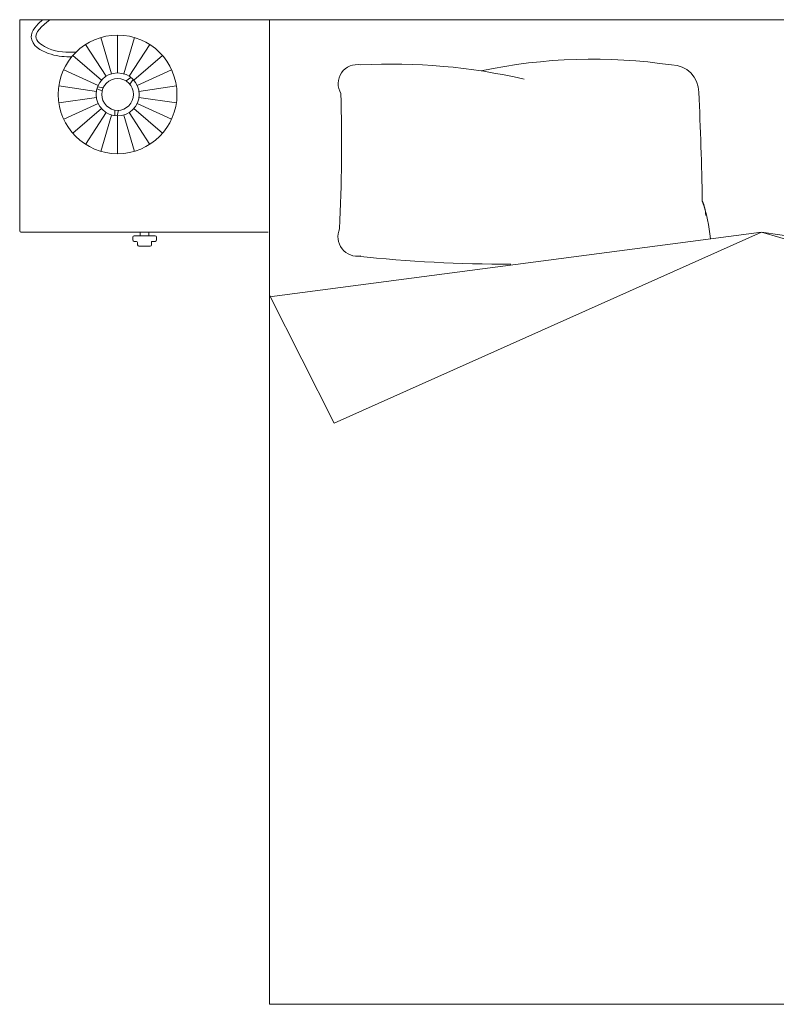
# Model space of a CAD drawing. Units: inches. Extents: x 1994 to 3075, y 3517 to 3950.
# Tile 7 of 58: x 1993.99644 to 1994.05149, y 3553.70967 to 3553.78125. Entities that reach past the tile are written whole.
import ezdxf

# ---------------------------------------------------------------- set-up
doc = ezdxf.new("R2010")
doc.units = ezdxf.units.IN
doc.layers.add('A-FURN-REFR', color=8, linetype='Continuous', lineweight=13)

msp = doc.modelspace()

# ---------------------------------------------------------------- linework, layer by layer
at = {"layer": 'A-FURN-REFR'}
for p, q in [((1994.014615338393, 3553.781253037129), (1993.996442127212, 3553.781253037129)), ((1993.996442127212, 3553.781253037129), (1993.996442127212, 3553.76590291077)), ((1994.014615338393, 3553.781253037129), (1993.996442127212, 3553.781253037129)), ((1994.014615338393, 3553.709671075784), (1994.014615338393, 3553.781253037129)), ((1994.014615338393, 3553.781253037129), (1994.050406319066, 3553.781253037129)), ((1994.014615338393, 3553.781253037129), (1994.086197299739, 3553.781253037129)), ((1994.014615338393, 3553.781253037129), (1994.014615338393, 3553.76590291077)), ((1994.00235315096, 3553.77996234353), (1994.003128737442, 3553.77732093855)), ((1994.003569221938, 3553.78013718814), (1994.003569221938, 3553.777384270659)), ((1994.003569221938, 3553.78013718814), (1994.003569221938, 3553.777384270659)), ((1994.004785292916, 3553.77996234353), (1994.004009706435, 3553.77732093855)), ((1994.001235598821, 3553.779451974569), (1994.002723938379, 3553.777136073012)), ((1994.004414505497, 3553.777136073012), (1994.005902845055, 3553.779451974569)), ((1994.000307102949, 3553.778647428315), (1994.002387619163, 3553.776844650753)), ((1994.004750824713, 3553.776844650753), (1994.006831340928, 3553.778647428315)), ((1993.999642884556, 3553.777613884321), (1994.002147026377, 3553.776470281071)), ((1994.004991417499, 3553.776470281071), (1994.007495559321, 3553.777613884321)), ((1994.004181245476, 3553.776804389888), (1994.00453887159, 3553.777047270305)), ((1994.004463846971, 3553.776556785599), (1994.004688097723, 3553.776912848794)), ((1993.999296754667, 3553.776435074175), (1994.002021651418, 3553.77604329317)), ((1994.002437874211, 3553.776069987851), (1994.002061906506, 3553.776236098163)), ((1994.002517003329, 3553.776305435665), (1994.002106774192, 3553.776373715132)), ((1994.005116792459, 3553.77604329317), (1994.007841689209, 3553.776435074175)), ((1993.999296754667, 3553.775206498065), (1994.002021651418, 3553.775598279071)), ((1994.005116792459, 3553.775598279071), (1994.007841689209, 3553.775206498065)), ((1993.999642884556, 3553.774027687919), (1994.002147026377, 3553.77517129117)), ((1994.000307102949, 3553.772994143925), (1994.002387619163, 3553.774796921488)), ((1994.003358659067, 3553.77468161429), (1994.003361507048, 3553.774271160867)), ((1994.003626943828, 3553.774663756577), (1994.003524948585, 3553.774257928554)), ((1994.004750824713, 3553.774796921488), (1994.006831340928, 3553.772994143925)), ((1994.004991417499, 3553.77517129117), (1994.007495559321, 3553.774027687919)), ((1994.001235598821, 3553.772189597672), (1994.002723938379, 3553.774505499229)), ((1994.003128737442, 3553.774320633691), (1994.00235315096, 3553.771679228711)), ((1994.003569221938, 3553.774257301582), (1994.003569221938, 3553.7715043841)), ((1994.003569221938, 3553.774257301582), (1994.003569221938, 3553.7715043841)), ((1994.004009706435, 3553.774320633691), (1994.004785292916, 3553.771679228711)), ((1994.004414505497, 3553.774505499229), (1994.005902845055, 3553.772189597672)), ((1993.99653663237, 3553.765808405612), (1994.014520833234, 3553.765808405612)), ((1994.004667007326, 3553.76544338097), (1994.004667007326, 3553.765232771723)), ((1994.006295953121, 3553.765537886128), (1994.004761512484, 3553.765537886128)), ((1994.005847638205, 3553.765808405612), (1994.0052098274, 3553.765808405612)), ((1994.0052098274, 3553.765808405612), (1994.0052098274, 3553.765537886128)), ((1994.005847638205, 3553.765537886128), (1994.005847638205, 3553.765808405612)), ((1994.006390458279, 3553.765232771723), (1994.006390458279, 3553.76544338097)), ((1994.050406319066, 3553.765802591595), (1994.014615338393, 3553.761110270129)), ((1994.019330692971, 3553.751926579221), (1994.050406319066, 3553.765802591595)), ((1994.08200406422, 3553.75649981287), (1994.050406319066, 3553.765802591595)), ((1994.050406319066, 3553.765802591595), (1994.086197299739, 3553.760685088365)), ((1994.004761512484, 3553.765138266565), (1994.004929071149, 3553.765138266565)), ((1994.005023576307, 3553.765043761406), (1994.005023576307, 3553.764886505597)), ((1994.005118081465, 3553.764792000439), (1994.005939384139, 3553.764792000439)), ((1994.006033889298, 3553.764886505597), (1994.006033889298, 3553.765138266565)), ((1994.006033889298, 3553.765138266565), (1994.006295953121, 3553.765138266565)), ((1994.014615338393, 3553.761226597718), (1994.019330692971, 3553.751926579221)), ((1994.050406319066, 3553.709671075784), (1994.014615338393, 3553.709671075784)), ((1994.050406319066, 3553.709671075784), (1994.086197299739, 3553.709671075784))]:
    msp.add_line(p, q, dxfattribs=at)
for radius in [0.0043164020201009, 0.0015634845390022, 0.0011584684638608]:
    msp.add_circle((1994.003569221938, 3553.77582078612), radius, dxfattribs=at)
for centre, radius, start, end in [((1994.038126880781, 3553.73972746297), 0.0386604856292291, 81.47022635647696, 102.1032641982298), ((1994.038126880781, 3553.73972746297), 0.0386604856292291, 81.47022635647696, 102.1032641982298), ((1994.020987024835, 3553.776609501392), 0.0013773909862166, 78.72778623498706, 211.6094986857782), ((1994.020987024835, 3553.776609501392), 0.0013773909862166, 78.72778623498706, 211.6094986857782), ((1994.023538440614, 3553.735112560259), 0.0429084957526809, 77.05638185161688, 93.04883220562752), ((1994.023538440614, 3553.735112560259), 0.0429084957526809, 77.05638185161688, 93.04883220562752), ((1994.043861132802, 3553.775978255031), 0.0019820668821378, 0, 90), ((1994.043861132802, 3553.775978255031), 0.0019820668821378, 0, 90), ((1993.81008941336, 3553.764307468219), 0.2360424856482679, 0.9125644663952034, 2.834064295864955), ((1993.81008941336, 3553.764307468219), 0.2360424856482679, 0.9125644663952034, 2.834064295864955), ((1993.877953801781, 3553.772411291119), 0.1419027684597849, 357.4333292641344, 1.403751564921032), ((1993.877953801781, 3553.772411291119), 0.1419027684597849, 357.4333292641344, 1.403751564921032), ((1994.043514142667, 3553.766894327521), 0.0028410445555686, 2.669769842706013, 24.37436785420747), ((1994.034287062718, 3553.764054157699), 0.0124777100514353, 5.86256739873855, 18.75888339460107), ((1994.021017191611, 3553.765479446885), 0.0014250910037829, 156.1084115545774, 279.6575795622506), ((1994.021017191611, 3553.765479446885), 0.0014250910037829, 156.1084115545774, 279.6575795622506), ((1993.99653663237, 3553.76590291077), 9.45051583805e-05, 180, 270), ((1994.004761512484, 3553.76544338097), 9.45051583805e-05, 90, 180), ((1994.004761512484, 3553.765232771723), 9.45051583805e-05, 180, 270), ((1994.006295953121, 3553.76544338097), 9.45051583805e-05, 0, 90), ((1994.006295953121, 3553.765232771723), 9.45051583805e-05, 270, 0), ((1994.004929071149, 3553.765043761406), 9.45051583805e-05, 0, 90), ((1994.005118081465, 3553.764886505597), 9.45051583805e-05, 180, 270), ((1994.005939384139, 3553.764886505597), 9.45051583805e-05, 270, 0), ((1994.032342052687, 3553.873903662037), 0.1104315287461407, 264.1139139330622, 269.9157410553413), ((1994.032342052687, 3553.873903662037), 0.1104315287461407, 264.1139139330622, 269.9157410553413)]:
    msp.add_arc(centre, radius, start, end, dxfattribs=at)
for points, knots in [([(1994.000231579868, 3553.778557841438), (1993.999759330298, 3553.778553992103), (1993.999258092903, 3553.778574259315), (1993.998191443662, 3553.778907428329), (1993.99751936082, 3553.779159156177), (1993.997157586806, 3553.780313714741), (1993.997557556096, 3553.78073398885), (1993.998003175492, 3553.781141867933), (1993.998066767109, 3553.781197724685), (1993.998131281946, 3553.781253037129)], [0.0077183477163671, 0.0077183477163671, 0.0077183477163671, 0.0077183477163671, 0.0428867239757183, 0.0428867239757183, 0.0785443346356031, 0.0785443346356031, 0.1084777623087474, 0.1084777623087474, 0.1132872864949097, 0.1132872864949097, 0.1132872864949097, 0.1132872864949097]), ([(1994.000532222368, 3553.778888025924), (1993.999878973019, 3553.778875793347), (1993.99885650102, 3553.778868956394), (1993.99712934616, 3553.779993483352), (1993.998073037213, 3553.780785400519), (1993.998638486558, 3553.781253037129)], [0, 0, 0, 0, 0.0020194675196073, 0.0031659294013192, 0.0048546887779338, 0.0048546887779338, 0.0048546887779338, 0.0048546887779338])]:
    msp.add_open_spline(points, degree=3, knots=knots, dxfattribs=at)

doc.saveas('drawing.dxf')
